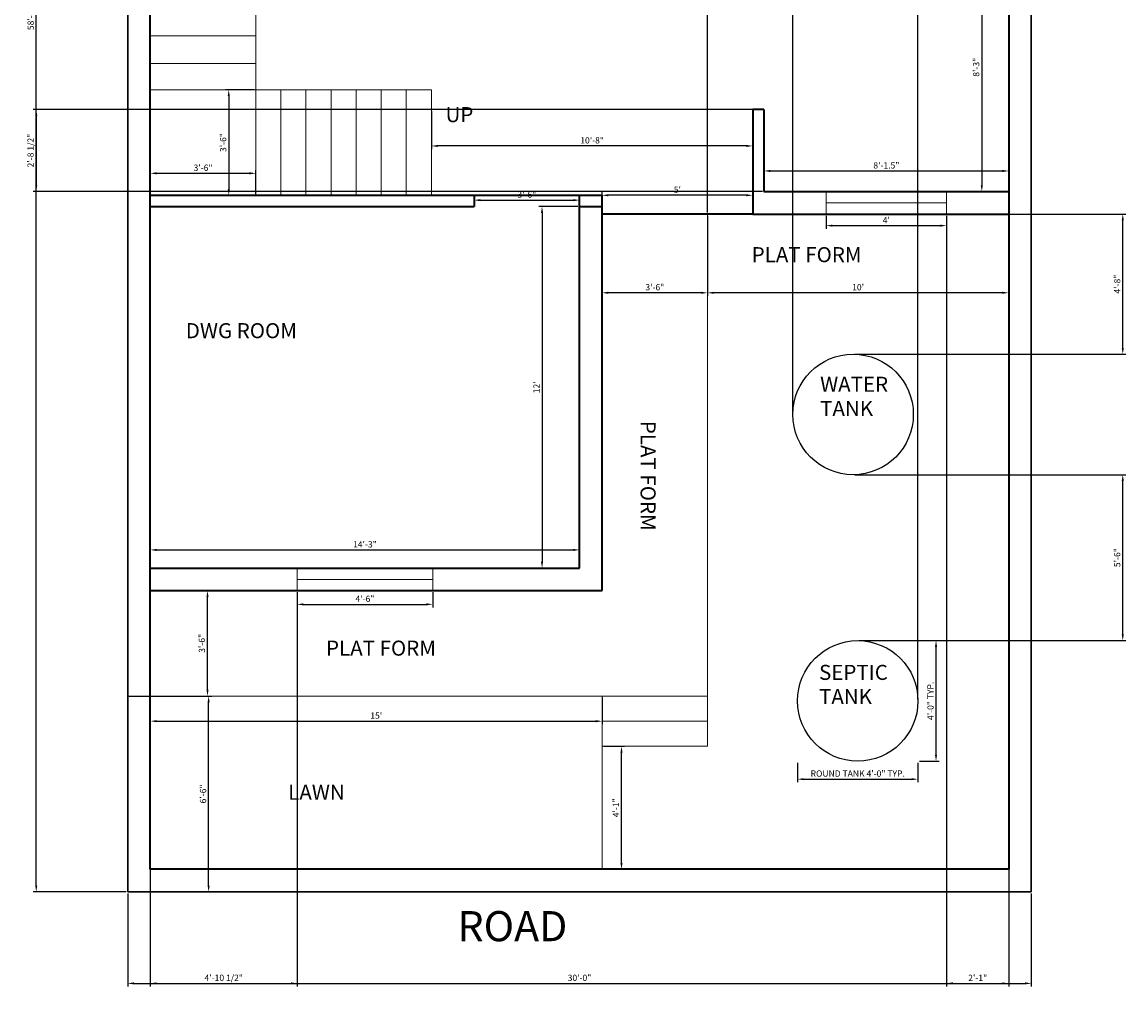
# Model space of a CAD drawing. Units: inches. Extents: x 2279 to 2719, y 394 to 1171.
# Tile 1 of 3: x 2279 to 2719, y 394 to 779. Entities that reach past the tile are written whole.
import ezdxf

# ---------------------------------------------------------------- set-up
doc = ezdxf.new("R2010")
doc.units = ezdxf.units.IN
for name, color, linetype, lineweight in [('A-ANNO-DIMS', 2, 'Continuous', 13), ('A-ANNO-TEXT', 7, 'Continuous', 18), ('A-AREA-IDEN', 7, 'Continuous', 25), ('A-FLOR-STRS', 3, 'Continuous', 20), ('A-GLAZ', 4, 'Continuous', 18), ('A-WALL', 7, 'Continuous', 35), ('C-PROP', 7, 'Continuous', 30), ('L-HRDS', 32, 'Continuous', 20), ('P-EQPM-TANK', 151, 'Continuous', 25)]:
    doc.layers.add(name, color=color, linetype=linetype, lineweight=lineweight)
doc.styles.get("Standard").update_dxf_attribs({"font": 'arial.ttf'})
doc.dimstyles.new('ISO-25', dxfattribs={"dimtxt": 2.5, "dimasz": 2.5, "dimexe": 1.25, "dimexo": 0.625, "dimtad": 1, "dimdec": 1, "dimlunit": 3, "dimtxsty": 'Standard', "dimcen": 2.5, "dimadec": 0, "dimazin": 0, "dimtfac": 1, "dimtdec": 1, "dimtmove": 0, "dimatfit": 3, "dimfxl": 1, "dimarcsym": 0})

# ---------------------------------------------------------------- blocks, each defined once
blk = doc.blocks.new('*D22')
at = {"layer": 'A-ANNO-DIMS', "color": 0, "lineweight": -2, "transparency": 16777216}
for p, q in [((2371.52, 751.95), (2360.14, 751.95)), ((2361.39, 749.45), (2361.39, 712.45)), ((2371.52, 709.95), (2360.14, 709.95))]:
    blk.add_line(p, q, dxfattribs=at)
at = {"layer": 'A-ANNO-DIMS', "color": 0, "transparency": 16777216}
for points in [[(2360.97, 749.45), (2361.8, 749.45), (2361.39, 751.95)], [(2360.97, 712.45), (2361.8, 712.45), (2361.39, 709.95)]]:
    blk.add_solid(points, dxfattribs=at)
at = {"layer": 'Defpoints', "color": 0, "transparency": 16777216}
for p in [(2372.14, 751.95), (2361.39, 709.95), (2372.14, 709.95)]:
    blk.add_point(p, dxfattribs=at)
at = {"layer": 'A-ANNO-DIMS', "color": 0, "transparency": 16777216, "insert": (2359.48, 730.95), "char_height": 2.5, "attachment_point": 5, "rotation": 90}
blk.add_mtext('3\'-6"', dxfattribs=at)
blk = doc.blocks.new('*D23')
at = {"layer": 'A-ANNO-DIMS', "color": 0, "lineweight": -2, "transparency": 16777216}
for p, q in [((2330.14, 710.58), (2330.14, 719.96)), ((2332.64, 718.71), (2369.64, 718.71)), ((2372.14, 710.58), (2372.14, 719.96))]:
    blk.add_line(p, q, dxfattribs=at)
at = {"layer": 'A-ANNO-DIMS', "color": 0, "transparency": 16777216}
for points in [[(2332.64, 719.12), (2332.64, 718.29), (2330.14, 718.71)], [(2369.64, 719.12), (2369.64, 718.29), (2372.14, 718.71)]]:
    blk.add_solid(points, dxfattribs=at)
at = {"layer": 'Defpoints', "color": 0, "transparency": 16777216}
for p in [(2372.14, 718.71), (2330.14, 709.95), (2372.14, 709.95)]:
    blk.add_point(p, dxfattribs=at)
at = {"layer": 'A-ANNO-DIMS', "color": 0, "transparency": 16777216, "insert": (2351.14, 720.61), "char_height": 2.5, "attachment_point": 5}
blk.add_mtext('3\'-6"', dxfattribs=at)
blk = doc.blocks.new('*D24')
at = {"layer": 'A-ANNO-DIMS', "color": 0, "lineweight": -2, "transparency": 16777216}
for p, q in [((2500.52, 705.45), (2484.96, 705.45)), ((2486.21, 702.95), (2486.21, 563.95)), ((2500.52, 561.45), (2484.96, 561.45))]:
    blk.add_line(p, q, dxfattribs=at)
at = {"layer": 'A-ANNO-DIMS', "color": 0, "transparency": 16777216}
for points in [[(2485.79, 702.95), (2486.63, 702.95), (2486.21, 705.45)], [(2485.79, 563.95), (2486.63, 563.95), (2486.21, 561.45)]]:
    blk.add_solid(points, dxfattribs=at)
at = {"layer": 'Defpoints', "color": 0, "transparency": 16777216}
for p in [(2501.14, 705.45), (2486.21, 561.45), (2501.14, 561.45)]:
    blk.add_point(p, dxfattribs=at)
at = {"layer": 'A-ANNO-DIMS', "color": 0, "transparency": 16777216, "insert": (2484.33, 633.45), "char_height": 2.5, "attachment_point": 5, "rotation": 90}
blk.add_mtext("12'", dxfattribs=at)
blk = doc.blocks.new('*D25')
at = {"layer": 'A-ANNO-DIMS', "color": 0, "lineweight": -2, "transparency": 16777216}
for p, q in [((2330.14, 562.08), (2330.14, 569.93)), ((2332.64, 568.68), (2498.64, 568.68)), ((2501.14, 562.08), (2501.14, 569.93))]:
    blk.add_line(p, q, dxfattribs=at)
at = {"layer": 'A-ANNO-DIMS', "color": 0, "transparency": 16777216}
for points in [[(2332.64, 569.09), (2332.64, 568.26), (2330.14, 568.68)], [(2498.64, 569.09), (2498.64, 568.26), (2501.14, 568.68)]]:
    blk.add_solid(points, dxfattribs=at)
at = {"layer": 'Defpoints', "color": 0, "transparency": 16777216}
for p in [(2501.14, 568.68), (2330.14, 561.45), (2501.14, 561.45)]:
    blk.add_point(p, dxfattribs=at)
at = {"layer": 'A-ANNO-DIMS', "color": 0, "transparency": 16777216, "insert": (2415.64, 570.58), "char_height": 2.5, "attachment_point": 5}
blk.add_mtext('14\'-3"', dxfattribs=at)
blk = doc.blocks.new('*D26')
at = {"layer": 'A-ANNO-DIMS', "color": 0, "lineweight": -2, "transparency": 16777216}
for p, q in [((2510.14, 701.83), (2510.14, 669.86)), ((2552.14, 701.83), (2552.14, 669.86)), ((2549.64, 671.11), (2512.64, 671.11))]:
    blk.add_line(p, q, dxfattribs=at)
at = {"layer": 'A-ANNO-DIMS', "color": 0, "transparency": 16777216}
for points in [[(2512.64, 671.53), (2512.64, 670.69), (2510.14, 671.11)], [(2549.64, 671.53), (2549.64, 670.69), (2552.14, 671.11)]]:
    blk.add_solid(points, dxfattribs=at)
at = {"layer": 'Defpoints', "color": 0, "transparency": 16777216}
for p in [(2510.14, 702.45), (2552.14, 702.45), (2510.14, 671.11)]:
    blk.add_point(p, dxfattribs=at)
at = {"layer": 'A-ANNO-DIMS', "color": 0, "transparency": 16777216, "insert": (2531.14, 673.01), "char_height": 2.5, "attachment_point": 5}
blk.add_mtext('3\'-6"', dxfattribs=at)
blk = doc.blocks.new('*D27')
at = {"layer": 'A-ANNO-DIMS', "color": 0, "lineweight": -2, "transparency": 16777216}
for p, q in [((2552.14, 701.83), (2552.14, 669.86)), ((2672.14, 701.83), (2672.14, 669.86)), ((2669.64, 671.11), (2554.64, 671.11))]:
    blk.add_line(p, q, dxfattribs=at)
at = {"layer": 'A-ANNO-DIMS', "color": 0, "transparency": 16777216}
for points in [[(2554.64, 671.53), (2554.64, 670.69), (2552.14, 671.11)], [(2669.64, 671.53), (2669.64, 670.69), (2672.14, 671.11)]]:
    blk.add_solid(points, dxfattribs=at)
at = {"layer": 'Defpoints', "color": 0, "transparency": 16777216}
for p in [(2552.14, 702.45), (2672.14, 702.45), (2552.14, 671.11)]:
    blk.add_point(p, dxfattribs=at)
at = {"layer": 'A-ANNO-DIMS', "color": 0, "transparency": 16777216, "insert": (2612.14, 673.01), "char_height": 2.5, "attachment_point": 5}
blk.add_mtext("10'", dxfattribs=at)
blk = doc.blocks.new('*D28')
at = {"layer": 'A-ANNO-DIMS', "color": 0, "lineweight": -2, "transparency": 16777216}
for p, q in [((2510.77, 490.45), (2519.11, 490.45)), ((2517.86, 443.95), (2517.86, 487.95)), ((2510.77, 441.45), (2519.11, 441.45))]:
    blk.add_line(p, q, dxfattribs=at)
at = {"layer": 'A-ANNO-DIMS', "color": 0, "transparency": 16777216}
for points in [[(2517.45, 487.95), (2518.28, 487.95), (2517.86, 490.45)], [(2517.45, 443.95), (2518.28, 443.95), (2517.86, 441.45)]]:
    blk.add_solid(points, dxfattribs=at)
at = {"layer": 'Defpoints', "color": 0, "transparency": 16777216}
for p in [(2510.14, 490.45), (2517.86, 490.45), (2510.14, 441.45)]:
    blk.add_point(p, dxfattribs=at)
at = {"layer": 'A-ANNO-DIMS', "color": 0, "transparency": 16777216, "insert": (2515.98, 465.95), "char_height": 2.5, "attachment_point": 5, "rotation": 90}
blk.add_mtext('4\'-1"', dxfattribs=at)
blk = doc.blocks.new('*D29')
at = {"layer": 'A-ANNO-DIMS', "color": 0, "lineweight": -2, "transparency": 16777216}
for p, q in [((2321.77, 510.45), (2354.62, 510.45)), ((2353.37, 434.95), (2353.37, 507.95)), ((2321.77, 432.45), (2354.62, 432.45))]:
    blk.add_line(p, q, dxfattribs=at)
at = {"layer": 'A-ANNO-DIMS', "color": 0, "transparency": 16777216}
for points in [[(2352.96, 507.95), (2353.79, 507.95), (2353.37, 510.45)], [(2352.96, 434.95), (2353.79, 434.95), (2353.37, 432.45)]]:
    blk.add_solid(points, dxfattribs=at)
at = {"layer": 'Defpoints', "color": 0, "transparency": 16777216}
for p in [(2321.14, 510.45), (2353.37, 510.45), (2321.14, 432.45)]:
    blk.add_point(p, dxfattribs=at)
at = {"layer": 'A-ANNO-DIMS', "color": 0, "transparency": 16777216, "insert": (2351.47, 471.45), "char_height": 2.5, "attachment_point": 5, "rotation": 90}
blk.add_mtext('6\'-6"', dxfattribs=at)
blk = doc.blocks.new('*D30')
at = {"layer": 'A-ANNO-DIMS', "color": 0, "lineweight": -2, "transparency": 16777216}
for p, q in [((2330.14, 509.83), (2330.14, 499.2)), ((2510.14, 509.83), (2510.14, 499.2)), ((2332.64, 500.45), (2507.64, 500.45))]:
    blk.add_line(p, q, dxfattribs=at)
at = {"layer": 'A-ANNO-DIMS', "color": 0, "transparency": 16777216}
for points in [[(2332.64, 500.87), (2332.64, 500.03), (2330.14, 500.45)], [(2507.64, 500.87), (2507.64, 500.03), (2510.14, 500.45)]]:
    blk.add_solid(points, dxfattribs=at)
at = {"layer": 'Defpoints', "color": 0, "transparency": 16777216}
for p in [(2330.14, 510.45), (2510.14, 510.45), (2510.14, 500.45)]:
    blk.add_point(p, dxfattribs=at)
at = {"layer": 'A-ANNO-DIMS', "color": 0, "transparency": 16777216, "insert": (2420.14, 502.35), "char_height": 2.5, "attachment_point": 5}
blk.add_mtext("15'", dxfattribs=at)
blk = doc.blocks.new('*D33')
at = {"layer": 'A-ANNO-DIMS', "color": 0, "lineweight": -2, "transparency": 16777216}
for p, q in [((2442.14, 743.43), (2442.14, 728.35)), ((2570.14, 743.43), (2570.14, 728.35)), ((2567.64, 729.6), (2444.64, 729.6))]:
    blk.add_line(p, q, dxfattribs=at)
at = {"layer": 'A-ANNO-DIMS', "color": 0, "transparency": 16777216}
for points in [[(2444.64, 730.02), (2444.64, 729.19), (2442.14, 729.6)], [(2567.64, 730.02), (2567.64, 729.19), (2570.14, 729.6)]]:
    blk.add_solid(points, dxfattribs=at)
at = {"layer": 'Defpoints', "color": 0, "transparency": 16777216}
for p in [(2442.14, 744.06), (2570.14, 744.06), (2442.14, 729.6)]:
    blk.add_point(p, dxfattribs=at)
at = {"layer": 'A-ANNO-DIMS', "color": 0, "transparency": 16777216, "insert": (2506.14, 731.51), "char_height": 2.5, "attachment_point": 5}
blk.add_mtext('10\'-8"', dxfattribs=at)
blk = doc.blocks.new('*D38')
at = {"layer": 'A-ANNO-DIMS', "color": 0, "lineweight": -2, "transparency": 16777216}
for p, q in [((2510.14, 703.08), (2510.14, 711.2)), ((2567.64, 709.95), (2512.64, 709.95)), ((2570.14, 703.08), (2570.14, 711.2))]:
    blk.add_line(p, q, dxfattribs=at)
at = {"layer": 'A-ANNO-DIMS', "color": 0, "transparency": 16777216}
for points in [[(2512.64, 710.37), (2512.64, 709.53), (2510.14, 709.95)], [(2567.64, 710.37), (2567.64, 709.53), (2570.14, 709.95)]]:
    blk.add_solid(points, dxfattribs=at)
at = {"layer": 'Defpoints', "color": 0, "transparency": 16777216}
for p in [(2510.14, 709.95), (2510.14, 702.45), (2570.14, 702.45)]:
    blk.add_point(p, dxfattribs=at)
at = {"layer": 'A-ANNO-DIMS', "color": 0, "transparency": 16777216, "insert": (2540.14, 711.85), "char_height": 2.5, "attachment_point": 5}
blk.add_mtext("5'", dxfattribs=at)
blk = doc.blocks.new('*U37')
for p, q in [((0, 100), (0, 0)), ((900, 100), (900, 0)), ((0, 50), (900, 50))]:
    blk.add_line(p, q)
blk = doc.blocks.new('*D44')
at = {"layer": 'A-ANNO-DIMS', "color": 0, "lineweight": -2, "transparency": 16777216}
for p, q in [((2459.14, 709.33), (2459.14, 706.76)), ((2501.14, 709.33), (2501.14, 706.76)), ((2461.64, 708.01), (2498.64, 708.01))]:
    blk.add_line(p, q, dxfattribs=at)
at = {"layer": 'A-ANNO-DIMS', "color": 0, "transparency": 16777216}
for points in [[(2461.64, 708.43), (2461.64, 707.59), (2459.14, 708.01)], [(2498.64, 708.43), (2498.64, 707.59), (2501.14, 708.01)]]:
    blk.add_solid(points, dxfattribs=at)
at = {"layer": 'Defpoints', "color": 0, "transparency": 16777216}
for p in [(2459.14, 709.95), (2501.14, 709.95), (2501.14, 708.01)]:
    blk.add_point(p, dxfattribs=at)
at = {"layer": 'A-ANNO-DIMS', "color": 0, "transparency": 16777216, "insert": (2480.14, 709.91), "char_height": 2.5, "attachment_point": 5}
blk.add_mtext('3\'-6"', dxfattribs=at)
blk = doc.blocks.new('*D45')
at = {"layer": 'A-ANNO-DIMS', "color": 0, "lineweight": -2, "transparency": 16777216}
for p, q in [((2388.64, 551.83), (2388.64, 545.74)), ((2442.64, 551.83), (2442.64, 545.74)), ((2391.14, 546.99), (2440.14, 546.99))]:
    blk.add_line(p, q, dxfattribs=at)
at = {"layer": 'A-ANNO-DIMS', "color": 0, "transparency": 16777216}
for points in [[(2391.14, 547.41), (2391.14, 546.58), (2388.64, 546.99)], [(2440.14, 547.41), (2440.14, 546.58), (2442.64, 546.99)]]:
    blk.add_solid(points, dxfattribs=at)
at = {"layer": 'Defpoints', "color": 0, "transparency": 16777216}
for p in [(2388.64, 552.45), (2442.64, 552.45), (2442.64, 546.99)]:
    blk.add_point(p, dxfattribs=at)
at = {"layer": 'A-ANNO-DIMS', "color": 0, "transparency": 16777216, "insert": (2415.64, 548.9), "char_height": 2.5, "attachment_point": 5}
blk.add_mtext('4\'-6"', dxfattribs=at)
blk = doc.blocks.new('*D46')
at = {"layer": 'A-ANNO-DIMS', "color": 0, "lineweight": -2, "transparency": 16777216}
for p, q in [((2599.39, 701.83), (2599.39, 696.61)), ((2647.39, 701.83), (2647.39, 696.61)), ((2601.89, 697.86), (2644.89, 697.86))]:
    blk.add_line(p, q, dxfattribs=at)
at = {"layer": 'A-ANNO-DIMS', "color": 0, "transparency": 16777216}
for points in [[(2601.89, 698.28), (2601.89, 697.45), (2599.39, 697.86)], [(2644.89, 698.28), (2644.89, 697.45), (2647.39, 697.86)]]:
    blk.add_solid(points, dxfattribs=at)
at = {"layer": 'Defpoints', "color": 0, "transparency": 16777216}
for p in [(2599.39, 702.45), (2647.39, 702.45), (2647.39, 697.86)]:
    blk.add_point(p, dxfattribs=at)
at = {"layer": 'A-ANNO-DIMS', "color": 0, "transparency": 16777216, "insert": (2623.39, 699.74), "char_height": 2.5, "attachment_point": 5}
blk.add_mtext("4'", dxfattribs=at)
blk = doc.blocks.new('*D47')
at = {"layer": 'A-ANNO-DIMS', "color": 0, "lineweight": -2, "transparency": 16777216}
for p, q in [((2671.52, 810.45), (2660.17, 810.45)), ((2661.42, 807.95), (2661.42, 713.95)), ((2671.52, 711.45), (2660.17, 711.45))]:
    blk.add_line(p, q, dxfattribs=at)
at = {"layer": 'A-ANNO-DIMS', "color": 0, "transparency": 16777216}
for points in [[(2661.01, 807.95), (2661.84, 807.95), (2661.42, 810.45)], [(2661.01, 713.95), (2661.84, 713.95), (2661.42, 711.45)]]:
    blk.add_solid(points, dxfattribs=at)
at = {"layer": 'Defpoints', "color": 0, "transparency": 16777216}
for p in [(2672.14, 810.45), (2661.42, 711.45), (2672.14, 711.45)]:
    blk.add_point(p, dxfattribs=at)
at = {"layer": 'A-ANNO-DIMS', "color": 0, "transparency": 16777216, "insert": (2659.52, 760.95), "char_height": 2.5, "attachment_point": 5, "rotation": 90}
blk.add_mtext('8\'-3"', dxfattribs=at)
blk = doc.blocks.new('*D48')
at = {"layer": 'A-ANNO-DIMS', "color": 0, "lineweight": -2, "transparency": 16777216}
for p, q in [((2574.64, 712.08), (2574.64, 720.89)), ((2577.14, 719.64), (2669.64, 719.64)), ((2672.14, 712.08), (2672.14, 720.89))]:
    blk.add_line(p, q, dxfattribs=at)
at = {"layer": 'A-ANNO-DIMS', "color": 0, "transparency": 16777216}
for points in [[(2577.14, 720.06), (2577.14, 719.22), (2574.64, 719.64)], [(2669.64, 720.06), (2669.64, 719.22), (2672.14, 719.64)]]:
    blk.add_solid(points, dxfattribs=at)
at = {"layer": 'Defpoints', "color": 0, "transparency": 16777216}
for p in [(2672.14, 719.64), (2574.64, 711.45), (2672.14, 711.45)]:
    blk.add_point(p, dxfattribs=at)
at = {"layer": 'A-ANNO-DIMS', "color": 0, "transparency": 16777216, "insert": (2623.39, 721.54), "char_height": 2.5, "attachment_point": 5}
blk.add_mtext('8\'-1.5"', dxfattribs=at)
blk = doc.blocks.new('*D49')
at = {"layer": 'A-ANNO-DIMS', "color": 0, "lineweight": -2, "transparency": 16777216}
for p, q in [((2330.77, 552.45), (2354.17, 552.45)), ((2352.92, 512.95), (2352.92, 549.95)), ((2330.77, 510.45), (2354.17, 510.45))]:
    blk.add_line(p, q, dxfattribs=at)
at = {"layer": 'A-ANNO-DIMS', "color": 0, "transparency": 16777216}
for points in [[(2352.5, 549.95), (2353.33, 549.95), (2352.92, 552.45)], [(2352.5, 512.95), (2353.33, 512.95), (2352.92, 510.45)]]:
    blk.add_solid(points, dxfattribs=at)
at = {"layer": 'Defpoints', "color": 0, "transparency": 16777216}
for p in [(2330.14, 552.45), (2352.92, 552.45), (2330.14, 510.45)]:
    blk.add_point(p, dxfattribs=at)
at = {"layer": 'A-ANNO-DIMS', "color": 0, "transparency": 16777216, "insert": (2351.02, 531.45), "char_height": 2.5, "attachment_point": 5, "rotation": 90}
blk.add_mtext('3\'-6"', dxfattribs=at)
blk = doc.blocks.new('TANK-ROUND-48IN')
blk.add_circle((24, 24), 24)
blk = doc.blocks.new('*D51')
at = {"layer": 'A-ANNO-DIMS', "color": 0, "lineweight": -2, "transparency": 16777216}
for p, q in [((2587.98, 483.92), (2587.98, 476.09)), ((2635.98, 483.92), (2635.98, 476.09)), ((2590.48, 477.34), (2633.48, 477.34))]:
    blk.add_line(p, q, dxfattribs=at)
at = {"layer": 'A-ANNO-DIMS', "color": 0, "transparency": 16777216}
for points in [[(2590.48, 477.76), (2590.48, 476.93), (2587.98, 477.34)], [(2633.48, 477.76), (2633.48, 476.93), (2635.98, 477.34)]]:
    blk.add_solid(points, dxfattribs=at)
at = {"layer": 'Defpoints', "color": 0, "transparency": 16777216}
for p in [(2587.98, 484.54), (2635.98, 484.54), (2635.98, 477.34)]:
    blk.add_point(p, dxfattribs=at)
at = {"layer": 'A-ANNO-DIMS', "color": 0, "transparency": 16777216, "insert": (2611.98, 479.26), "char_height": 2.5, "attachment_point": 5}
blk.add_mtext('ROUND TANK 4\'-0" TYP.', dxfattribs=at)
blk = doc.blocks.new('*D52')
at = {"layer": 'A-ANNO-DIMS', "color": 0, "lineweight": -2, "transparency": 16777216}
for p, q in [((2636.6, 532.54), (2644.43, 532.54)), ((2643.18, 487.04), (2643.18, 530.04)), ((2636.6, 484.54), (2644.43, 484.54))]:
    blk.add_line(p, q, dxfattribs=at)
at = {"layer": 'A-ANNO-DIMS', "color": 0, "transparency": 16777216}
for points in [[(2642.76, 530.04), (2643.6, 530.04), (2643.18, 532.54)], [(2642.76, 487.04), (2643.6, 487.04), (2643.18, 484.54)]]:
    blk.add_solid(points, dxfattribs=at)
at = {"layer": 'Defpoints', "color": 0, "transparency": 16777216}
for p in [(2635.98, 532.54), (2643.18, 532.54), (2635.98, 484.54)]:
    blk.add_point(p, dxfattribs=at)
at = {"layer": 'A-ANNO-DIMS', "color": 0, "transparency": 16777216, "insert": (2641.28, 508.54), "char_height": 2.5, "attachment_point": 5, "rotation": 90}
blk.add_mtext('4\'-0" TYP.', dxfattribs=at)
blk = doc.blocks.new('*D53')
at = {"layer": 'A-ANNO-DIMS', "color": 0, "lineweight": -2, "transparency": 16777216}
for p, q in [((2552.14, 703.08), (2552.14, 1166.15)), ((2586.14, 623.28), (2586.14, 1166.15)), ((2583.64, 1164.9), (2554.64, 1164.9))]:
    blk.add_line(p, q, dxfattribs=at)
at = {"layer": 'A-ANNO-DIMS', "color": 0, "transparency": 16777216}
for points in [[(2554.64, 1165.32), (2554.64, 1164.48), (2552.14, 1164.9)], [(2583.64, 1165.32), (2583.64, 1164.48), (2586.14, 1164.9)]]:
    blk.add_solid(points, dxfattribs=at)
at = {"layer": 'Defpoints', "color": 0, "transparency": 16777216}
for p in [(2552.14, 1164.9), (2552.14, 702.45), (2586.14, 622.65)]:
    blk.add_point(p, dxfattribs=at)
at = {"layer": 'A-ANNO-DIMS', "color": 0, "transparency": 16777216, "insert": (2569.14, 1166.8), "char_height": 2.5, "attachment_point": 5}
blk.add_mtext('2\'-10"', dxfattribs=at)
blk = doc.blocks.new('*D54')
at = {"layer": 'A-ANNO-DIMS', "color": 0, "lineweight": -2, "transparency": 16777216}
for p, q in [((2600.02, 702.45), (2718.84, 702.45)), ((2717.59, 649.15), (2717.59, 699.95)), ((2610.77, 646.65), (2718.84, 646.65))]:
    blk.add_line(p, q, dxfattribs=at)
at = {"layer": 'A-ANNO-DIMS', "color": 0, "transparency": 16777216}
for points in [[(2717.17, 699.95), (2718.01, 699.95), (2717.59, 702.45)], [(2717.17, 649.15), (2718.01, 649.15), (2717.59, 646.65)]]:
    blk.add_solid(points, dxfattribs=at)
at = {"layer": 'Defpoints', "color": 0, "transparency": 16777216}
for p in [(2599.39, 702.45), (2717.59, 702.45), (2610.14, 646.65)]:
    blk.add_point(p, dxfattribs=at)
at = {"layer": 'A-ANNO-DIMS', "color": 0, "transparency": 16777216, "insert": (2715.69, 674.55), "char_height": 2.5, "attachment_point": 5, "rotation": 90}
blk.add_mtext('4\'-8"', dxfattribs=at)
blk = doc.blocks.new('*D55')
at = {"layer": 'A-ANNO-DIMS', "color": 0, "lineweight": -2, "transparency": 16777216}
for p, q in [((2635.98, 509.17), (2635.98, 1166.15)), ((2672.14, 442.08), (2672.14, 1166.15)), ((2638.48, 1164.9), (2669.64, 1164.9))]:
    blk.add_line(p, q, dxfattribs=at)
at = {"layer": 'A-ANNO-DIMS', "color": 0, "transparency": 16777216}
for points in [[(2638.48, 1165.32), (2638.48, 1164.48), (2635.98, 1164.9)], [(2669.64, 1165.32), (2669.64, 1164.48), (2672.14, 1164.9)]]:
    blk.add_solid(points, dxfattribs=at)
at = {"layer": 'Defpoints', "color": 0, "transparency": 16777216}
for p in [(2672.14, 1164.9), (2635.98, 508.54), (2672.14, 441.45)]:
    blk.add_point(p, dxfattribs=at)
at = {"layer": 'A-ANNO-DIMS', "color": 0, "transparency": 16777216, "insert": (2654.06, 1166.8), "char_height": 2.5, "attachment_point": 5}
blk.add_mtext('3\'-0"', dxfattribs=at)
blk = doc.blocks.new('*D56')
at = {"layer": 'A-ANNO-DIMS', "color": 0, "lineweight": -2, "transparency": 16777216}
for p, q in [((2610.77, 598.65), (2718.84, 598.65)), ((2717.59, 535.04), (2717.59, 596.15)), ((2612.6, 532.54), (2718.84, 532.54))]:
    blk.add_line(p, q, dxfattribs=at)
at = {"layer": 'A-ANNO-DIMS', "color": 0, "transparency": 16777216}
for points in [[(2717.17, 596.15), (2718.01, 596.15), (2717.59, 598.65)], [(2717.17, 535.04), (2718.01, 535.04), (2717.59, 532.54)]]:
    blk.add_solid(points, dxfattribs=at)
at = {"layer": 'Defpoints', "color": 0, "transparency": 16777216}
for p in [(2610.14, 598.65), (2717.59, 598.65), (2611.98, 532.54)]:
    blk.add_point(p, dxfattribs=at)
at = {"layer": 'A-ANNO-DIMS', "color": 0, "transparency": 16777216, "insert": (2715.69, 565.6), "char_height": 2.5, "attachment_point": 5, "rotation": 90}
blk.add_mtext('5\'-6"', dxfattribs=at)
blk = doc.blocks.new('*D63')
at = {"layer": 'A-ANNO-DIMS', "color": 0, "lineweight": -2, "transparency": 16777216}
for p, q in [((2574.02, 744.06), (2283.44, 744.06)), ((2284.69, 741.56), (2284.69, 713.95)), ((2574.02, 711.45), (2283.44, 711.45))]:
    blk.add_line(p, q, dxfattribs=at)
at = {"layer": 'A-ANNO-DIMS', "color": 0, "transparency": 16777216}
for points in [[(2284.27, 741.56), (2285.11, 741.56), (2284.69, 744.06)], [(2284.27, 713.95), (2285.11, 713.95), (2284.69, 711.45)]]:
    blk.add_solid(points, dxfattribs=at)
at = {"layer": 'Defpoints', "color": 0, "transparency": 16777216}
for p in [(2574.64, 744.06), (2284.69, 711.45), (2574.64, 711.45)]:
    blk.add_point(p, dxfattribs=at)
at = {"layer": 'A-ANNO-DIMS', "color": 0, "transparency": 16777216, "insert": (2282.77, 727.75), "char_height": 2.5, "attachment_point": 5, "rotation": 90}
blk.add_mtext('2\'-8 1/2"', dxfattribs=at)
blk = doc.blocks.new('*D64')
at = {"layer": 'A-ANNO-DIMS', "color": 0, "lineweight": -2, "transparency": 16777216}
for p, q in [((2330.14, 551.83), (2330.14, 394.75)), ((2388.64, 551.83), (2388.64, 394.75)), ((2332.64, 396), (2386.14, 396))]:
    blk.add_line(p, q, dxfattribs=at)
at = {"layer": 'A-ANNO-DIMS', "color": 0, "transparency": 16777216}
for points in [[(2332.64, 396.42), (2332.64, 395.58), (2330.14, 396)], [(2386.14, 396.42), (2386.14, 395.58), (2388.64, 396)]]:
    blk.add_solid(points, dxfattribs=at)
at = {"layer": 'Defpoints', "color": 0, "transparency": 16777216}
for p in [(2330.14, 552.45), (2388.64, 552.45), (2388.64, 396)]:
    blk.add_point(p, dxfattribs=at)
at = {"layer": 'A-ANNO-DIMS', "color": 0, "transparency": 16777216, "insert": (2359.39, 397.92), "char_height": 2.5, "attachment_point": 5}
blk.add_mtext('4\'-10 1/2"', dxfattribs=at)
blk = doc.blocks.new('*D65')
at = {"layer": 'A-ANNO-DIMS', "color": 0, "lineweight": -2, "transparency": 16777216}
for p, q in [((2647.39, 701.83), (2647.39, 394.75)), ((2672.14, 701.83), (2672.14, 394.75)), ((2649.89, 396), (2669.64, 396))]:
    blk.add_line(p, q, dxfattribs=at)
at = {"layer": 'A-ANNO-DIMS', "color": 0, "transparency": 16777216}
for points in [[(2649.89, 396.42), (2649.89, 395.58), (2647.39, 396)], [(2669.64, 396.42), (2669.64, 395.58), (2672.14, 396)]]:
    blk.add_solid(points, dxfattribs=at)
at = {"layer": 'Defpoints', "color": 0, "transparency": 16777216}
for p in [(2647.39, 702.45), (2672.14, 702.45), (2672.14, 396)]:
    blk.add_point(p, dxfattribs=at)
at = {"layer": 'A-ANNO-DIMS', "color": 0, "transparency": 16777216, "insert": (2659.77, 397.88), "char_height": 2.5, "attachment_point": 5}
blk.add_mtext('2\'-1"', dxfattribs=at)
blk = doc.blocks.new('*D67')
at = {"layer": 'A-ANNO-DIMS', "color": 0, "lineweight": -2, "transparency": 16777216}
for p, q in [((2321.14, 431.83), (2321.14, 394.75)), ((2681.14, 431.83), (2681.14, 394.75)), ((2323.64, 396), (2678.64, 396))]:
    blk.add_line(p, q, dxfattribs=at)
at = {"layer": 'A-ANNO-DIMS', "color": 0, "transparency": 16777216}
for points in [[(2323.64, 396.42), (2323.64, 395.58), (2321.14, 396)], [(2678.64, 396.42), (2678.64, 395.58), (2681.14, 396)]]:
    blk.add_solid(points, dxfattribs=at)
at = {"layer": 'Defpoints', "color": 0, "transparency": 16777216}
for p in [(2321.14, 432.45), (2681.14, 432.45), (2681.14, 396)]:
    blk.add_point(p, dxfattribs=at)
at = {"layer": 'A-ANNO-DIMS', "color": 0, "transparency": 16777216, "insert": (2501.14, 397.9), "char_height": 2.5, "attachment_point": 5}
blk.add_mtext('30\'-0"', dxfattribs=at)
blk = doc.blocks.new('*D68')
at = {"layer": 'A-ANNO-DIMS', "color": 0, "lineweight": -2, "transparency": 16777216}
for p, q in [((2320.52, 1128.45), (2283.44, 1128.45)), ((2284.69, 434.95), (2284.69, 1125.95)), ((2320.52, 432.45), (2283.44, 432.45))]:
    blk.add_line(p, q, dxfattribs=at)
at = {"layer": 'A-ANNO-DIMS', "color": 0, "transparency": 16777216}
for points in [[(2284.27, 1125.95), (2285.11, 1125.95), (2284.69, 1128.45)], [(2284.27, 434.95), (2285.11, 434.95), (2284.69, 432.45)]]:
    blk.add_solid(points, dxfattribs=at)
at = {"layer": 'Defpoints', "color": 0, "transparency": 16777216}
for p in [(2284.69, 1128.45), (2321.14, 1128.45), (2321.14, 432.45)]:
    blk.add_point(p, dxfattribs=at)
at = {"layer": 'A-ANNO-DIMS', "color": 0, "transparency": 16777216, "insert": (2282.79, 780.45), "char_height": 2.5, "attachment_point": 5, "rotation": 90}
blk.add_mtext('58\'-0"', dxfattribs=at)

msp = doc.modelspace()

# ---------------------------------------------------------------- linework, layer by layer
at = {"layer": 'A-FLOR-STRS'}
for p, q in [((2372.14, 870.45), (2372.14, 709.95)), ((2372.14, 773.45), (2330.14, 773.45)), ((2372.14, 762.45), (2330.14, 762.45)), ((2382.14, 751.95), (2330.14, 751.95)), ((2382.14, 751.95), (2382.14, 709.95)), ((2382.14, 751.95), (2442.14, 751.95)), ((2392.14, 751.95), (2392.14, 709.95)), ((2402.14, 751.95), (2402.14, 709.95)), ((2412.14, 751.95), (2412.14, 709.95)), ((2422.14, 751.95), (2422.14, 709.95)), ((2432.14, 751.95), (2432.14, 709.95)), ((2442.14, 751.95), (2442.14, 709.95)), ((2552.14, 500.45), (2510.14, 500.45)), ((2552.14, 490.45), (2510.14, 490.45))]:
    msp.add_line(p, q, dxfattribs=at)
at = {"layer": 'A-GLAZ'}
for p, q in [((2599.39, 711.45), (2599.39, 702.45)), ((2647.39, 702.45), (2647.39, 711.45)), ((2599.39, 702.45), (2647.39, 702.45)), ((2388.64, 552.45), (2388.64, 561.45)), ((2442.64, 561.45), (2442.64, 552.45)), ((2442.64, 552.45), (2388.64, 552.45))]:
    msp.add_line(p, q, dxfattribs=at)
at = {"layer": 'A-WALL'}
for p, q in [((2330.14, 552.45), (2330.14, 1119.45)), ((2672.14, 1119.45), (2672.14, 441.45)), ((2570.14, 744.06), (2570.14, 702.45)), ((2574.64, 744.06), (2570.14, 744.06)), ((2574.64, 744.06), (2574.64, 711.45)), ((2330.14, 709.95), (2510.14, 709.95)), ((2459.14, 709.95), (2459.14, 705.45)), ((2501.14, 561.45), (2501.14, 709.95)), ((2510.14, 702.45), (2510.14, 709.95)), ((2510.14, 552.45), (2510.14, 709.95)), ((2574.64, 711.45), (2672.14, 711.45)), ((2330.14, 705.45), (2459.14, 705.45)), ((2501.14, 705.45), (2510.14, 705.45)), ((2570.14, 702.45), (2510.14, 702.45)), ((2570.14, 702.45), (2672.14, 702.45)), ((2330.14, 561.45), (2501.14, 561.45)), ((2330.14, 441.45), (2330.14, 552.45)), ((2330.14, 552.45), (2510.14, 552.45)), ((2672.14, 441.45), (2330.14, 441.45))]:
    msp.add_line(p, q, dxfattribs=at)
at = {"layer": 'C-PROP'}
for p, q in [((2321.14, 552.45), (2321.14, 1128.45)), ((2681.14, 1128.45), (2681.14, 432.45)), ((2321.14, 432.45), (2321.14, 552.45)), ((2681.14, 432.45), (2321.14, 432.45))]:
    msp.add_line(p, q, dxfattribs=at)
at = {"layer": 'L-HRDS'}
for p, q in [((2552.14, 702.45), (2552.14, 490.45)), ((2552.14, 510.45), (2321.14, 510.45)), ((2510.14, 441.45), (2510.14, 510.45))]:
    msp.add_line(p, q, dxfattribs=at)

# ---------------------------------------------------------------- block references
at = {"layer": 'A-GLAZ'}
for p, xscale, yscale, zscale in [((2599.39, 704.28), 0.0533333333333332, 0.0533333333333332, 0.0533333333333332), ((2388.64, 553.95), 0.0599999999999998, 0.0599999999999998, 0.0599999999999998)]:
    msp.add_blockref('*U37', p, dxfattribs=dict(at, xscale=xscale, yscale=yscale, zscale=zscale))
at = {"layer": 'P-EQPM-TANK'}
for p in [(2586.14, 598.65), (2587.98, 484.54)]:
    msp.add_blockref('TANK-ROUND-48IN', p, dxfattribs=at)

# ---------------------------------------------------------------- texts
at = {"layer": 'A-ANNO-TEXT'}
for s, height, p in [('UP', 6, (2447.76, 739.09)), ('WATER ', 6, (2597.01, 631.66)), ('TANK', 6, (2597.01, 622.03)), ('SEPTIC ', 6, (2596.58, 516.89)), ('TANK', 6, (2596.58, 507.25)), ('ROAD', 12, (2452.54, 412.79))]:
    msp.add_text(s, height=height, dxfattribs=at).set_placement(p)
at = {"layer": 'A-AREA-IDEN'}
for s, p in [('PLAT FORM', (2569.74, 683.3)), ('DWG ROOM', (2344.27, 653.01)), ('PLAT FORM', (2400.15, 526.55)), ('LAWN', (2385.07, 469.12))]:
    msp.add_text(s, height=6, dxfattribs=at).set_placement(p)
msp.add_text('PLAT FORM', height=6, rotation=270, dxfattribs=at).set_placement((2525.46, 620.1))

# ---------------------------------------------------------------- dimensions: what is measured, and where the dimension line sits
at = {"layer": 'A-ANNO-DIMS'}
for base, p1, p2, override, picture, middle in [((2552.14, 1164.9), (2586.14, 622.65), (2552.14, 702.45), {"dimdec": 1, "dimlfac": 1, "dimrnd": 0, "dimzin": 1, "dimdsep": 46, "dimlunit": 4, "dimfrac": 2}, '*D53', (2569.14, 1166.8)), ((2672.14, 1164.9), (2635.98, 508.54), (2672.14, 441.45), {"dimdec": 1, "dimlfac": 1, "dimrnd": 0, "dimzin": 1, "dimdsep": 46, "dimlunit": 4, "dimfrac": 2}, '*D55', (2654.06, 1166.8)), ((2442.14, 729.6), (2570.14, 744.06), (2442.14, 744.06), {"dimclrd": 0, "dimclre": 0, "dimclrt": 0}, '*D33', (2506.14, 731.51)), ((2372.14, 718.71), (2330.14, 709.95), (2372.14, 709.95), {"dimclrd": 0, "dimclre": 0, "dimclrt": 0}, '*D23', (2351.14, 720.61)), ((2672.14, 719.64), (2574.64, 711.45), (2672.14, 711.45), {"dimclrd": 0, "dimclre": 0, "dimclrt": 0}, '*D48', (2623.39, 721.54)), ((2510.14, 709.95), (2570.14, 702.45), (2510.14, 702.45), {"dimclrd": 0, "dimclre": 0, "dimclrt": 0}, '*D38', (2540.14, 711.85)), ((2501.14, 708.01), (2459.14, 709.95), (2501.14, 709.95), {"dimclrd": 0, "dimclre": 0, "dimclrt": 0}, '*D44', (2480.14, 709.91)), ((2510.14, 671.11), (2552.14, 702.45), (2510.14, 702.45), {"dimclrd": 0, "dimclre": 0, "dimclrt": 0}, '*D26', (2531.14, 673.01)), ((2552.14, 671.11), (2672.14, 702.45), (2552.14, 702.45), {"dimclrd": 0, "dimclre": 0, "dimclrt": 0}, '*D27', (2612.14, 673.01)), ((2647.39, 697.86), (2599.39, 702.45), (2647.39, 702.45), {"dimclrd": 0, "dimclre": 0, "dimclrt": 0}, '*D46', (2623.39, 699.74)), ((2672.140465, 396.001042), (2647.390465, 702.451042), (2672.140465, 702.451042), {"dimdec": 1, "dimlfac": 1, "dimrnd": 0, "dimzin": 1, "dimdsep": 46, "dimlunit": 4, "dimfrac": 2}, '*D65', (2659.765465, 397.88115796)), ((2501.14, 568.68), (2330.14, 561.45), (2501.14, 561.45), {"dimclrd": 0, "dimclre": 0, "dimclrt": 0}, '*D25', (2415.64, 570.58)), ((2388.64, 396), (2330.14, 552.45), (2388.64, 552.45), {"dimdec": 1, "dimlfac": 1, "dimrnd": 0, "dimzin": 1, "dimdsep": 46, "dimlunit": 4, "dimfrac": 2}, '*D64', (2359.39, 397.92)), ((2442.64, 546.99), (2388.64, 552.45), (2442.64, 552.45), {"dimclrd": 0, "dimclre": 0, "dimclrt": 0}, '*D45', (2415.64, 548.9)), ((2510.14, 500.45), (2330.14, 510.45), (2510.14, 510.45), {"dimclrd": 0, "dimclre": 0, "dimclrt": 0}, '*D30', (2420.14, 502.35)), ((2681.14, 396), (2321.14, 432.45), (2681.14, 432.45), {"dimdec": 1, "dimlfac": 1, "dimrnd": 0, "dimzin": 1, "dimdsep": 46, "dimlunit": 4, "dimfrac": 2}, '*D67', (2501.14, 397.9))]:
    dim = msp.add_linear_dim(base=base, p1=p1, p2=p2, dimstyle='ISO-25', override=override, dxfattribs=at)
    dim.commit()
    dim.dimension.update_dxf_attribs({"geometry": picture, "text_midpoint": middle})
for base, p1, p2, override, picture, middle in [((2284.69, 1128.45), (2321.14, 432.45), (2321.14, 1128.45), {"dimdec": 1, "dimlfac": 1, "dimrnd": 0, "dimzin": 1, "dimdsep": 46, "dimlunit": 4, "dimfrac": 2}, '*D68', (2282.79, 780.45)), ((2661.42, 711.45), (2672.14, 810.45), (2672.14, 711.45), {"dimclrd": 0, "dimclre": 0, "dimclrt": 0}, '*D47', (2659.52, 760.95)), ((2361.39, 709.95), (2372.14, 751.95), (2372.14, 709.95), {"dimclrd": 0, "dimclre": 0, "dimclrt": 0}, '*D22', (2359.48, 730.95)), ((2284.69, 711.45), (2574.64, 744.06), (2574.64, 711.45), {"dimdec": 1, "dimlfac": 1, "dimrnd": 0, "dimzin": 1, "dimdsep": 46, "dimlunit": 4, "dimfrac": 2}, '*D63', (2282.77, 727.75)), ((2486.21, 561.45), (2501.14, 705.45), (2501.14, 561.45), {"dimclrd": 0, "dimclre": 0, "dimclrt": 0}, '*D24', (2484.33, 633.45)), ((2717.59, 702.45), (2610.14, 646.65), (2599.39, 702.45), {"dimdec": 1, "dimlfac": 1, "dimrnd": 0, "dimzin": 1, "dimdsep": 46, "dimlunit": 4, "dimfrac": 2}, '*D54', (2715.69, 674.55)), ((2717.59, 598.65), (2611.98, 532.54), (2610.14, 598.65), {"dimdec": 1, "dimlfac": 1, "dimrnd": 0, "dimzin": 1, "dimdsep": 46, "dimlunit": 4, "dimfrac": 2}, '*D56', (2715.69, 565.6)), ((2352.92, 552.45), (2330.14, 510.45), (2330.14, 552.45), {"dimclrd": 0, "dimclre": 0, "dimclrt": 0}, '*D49', (2351.02, 531.45)), ((2353.37, 510.45), (2321.14, 432.45), (2321.14, 510.45), {"dimclrd": 0, "dimclre": 0, "dimclrt": 0}, '*D29', (2351.47, 471.45)), ((2517.86, 490.45), (2510.14, 441.45), (2510.14, 490.45), {"dimclrd": 0, "dimclre": 0, "dimclrt": 0}, '*D28', (2515.98, 465.95))]:
    dim = msp.add_linear_dim(base=base, p1=p1, p2=p2, angle=90, dimstyle='ISO-25', override=override, dxfattribs=at)
    dim.commit()
    dim.dimension.update_dxf_attribs({"geometry": picture, "text_midpoint": middle})
dim = msp.add_linear_dim(base=(2643.18, 532.54), p1=(2635.98, 484.54), p2=(2635.98, 532.54), angle=90, text='<> TYP.', dimstyle='ISO-25', override={"dimdec": 1, "dimlfac": 1, "dimrnd": 0, "dimzin": 1, "dimdsep": 46, "dimlunit": 4, "dimfrac": 2}, dxfattribs=at)
dim.commit()
dim.dimension.update_dxf_attribs({"geometry": '*D52', "text_midpoint": (2641.28, 508.54)})
dim = msp.add_linear_dim(base=(2635.98, 477.34), p1=(2587.98, 484.54), p2=(2635.98, 484.54), text='ROUND TANK <> TYP.', dimstyle='ISO-25', override={"dimdec": 1, "dimlfac": 1, "dimrnd": 0, "dimzin": 1, "dimdsep": 46, "dimlunit": 4, "dimfrac": 2}, dxfattribs=at)
dim.commit()
dim.dimension.update_dxf_attribs({"geometry": '*D51', "text_midpoint": (2611.98, 479.26)})

doc.saveas('drawing.dxf')
